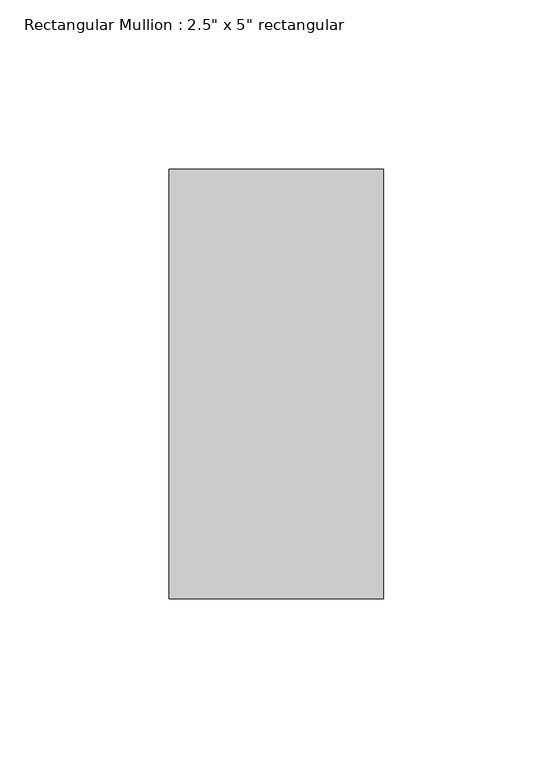
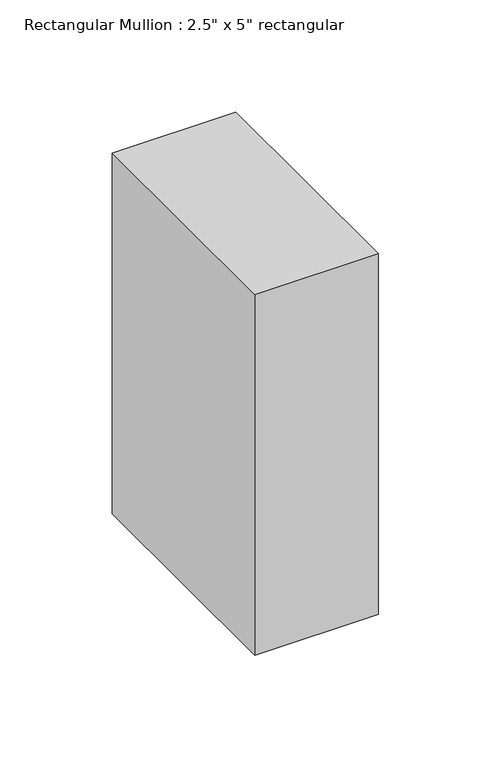
"""IFC4 building model written with IfcOpenShell, lengths in millimetres: member geometry."""

from ifc_helpers import new_model, si_unit, frame, origin, place, context, project, spatial, polyline, outline, extrude, source, transform, mapped, element, save


def member_fe2d9451(model_context):
    return source(origin(), model_context, "Body", "SweptSolid", [
        extrude(outline(polyline([(0.0, 63.5), (0.0, -63.5), (-63.5, -63.5), (-63.5, 63.5), (0.0, 63.5)])), frame((0.0, 0.0, -196.1049185), z_axis=(0.0, 0.0, 1.0), x_axis=(1.0, 0.0, 0.0)), (0.0, 0.0, 1.0), 196.1049185),
    ])


if __name__ == "__main__":
    model = new_model("IFC4")
    model_context = context("Model", 3, world=origin())
    ifc_project = project(units=[si_unit("LENGTHUNIT", "METRE", prefix="MILLI")], contexts=[model_context])
    site = spatial("IfcSite", under=ifc_project)
    building = spatial("IfcBuilding", under=site)
    placement = place(None, origin())
    member_shape = member_fe2d9451(model_context)
    element("IfcMember", 1, ObjectType="Rectangular Mullion : 2.5\" x 5\" rectangular", at=placement, inside=building, context=model_context, shape_type="MappedRepresentation", body=[
        mapped(member_shape, transform((0.0, 0.0, 0.0), x_axis=(1.0, 0.0, 0.0), y_axis=(0.0, 1.0, 0.0), z_axis=(0.0, 0.0, 1.0))),
    ])
    save(model, "model.ifc")

# Revit data of these elements
# Type "Rectangular Mullion : 2.5\" x 5\" rectangular"
#   built-in parameter 1007304 = 0.416667 (stored number, unit not read)
#   built-in parameter 1007301 = 0.104167 (stored number, unit not read)
#   built-in parameter 1007300 = 0.104167 (stored number, unit not read)
# Element 1 (IfcMember, "Rectangular Mullion : 2.5\" x 5\" rectangular")
#   Materials on its faces: "mullions"
# Materials
#   "mullions": class "Generic", colour RGB 120 120 120, transparency 0, Cost = 0
